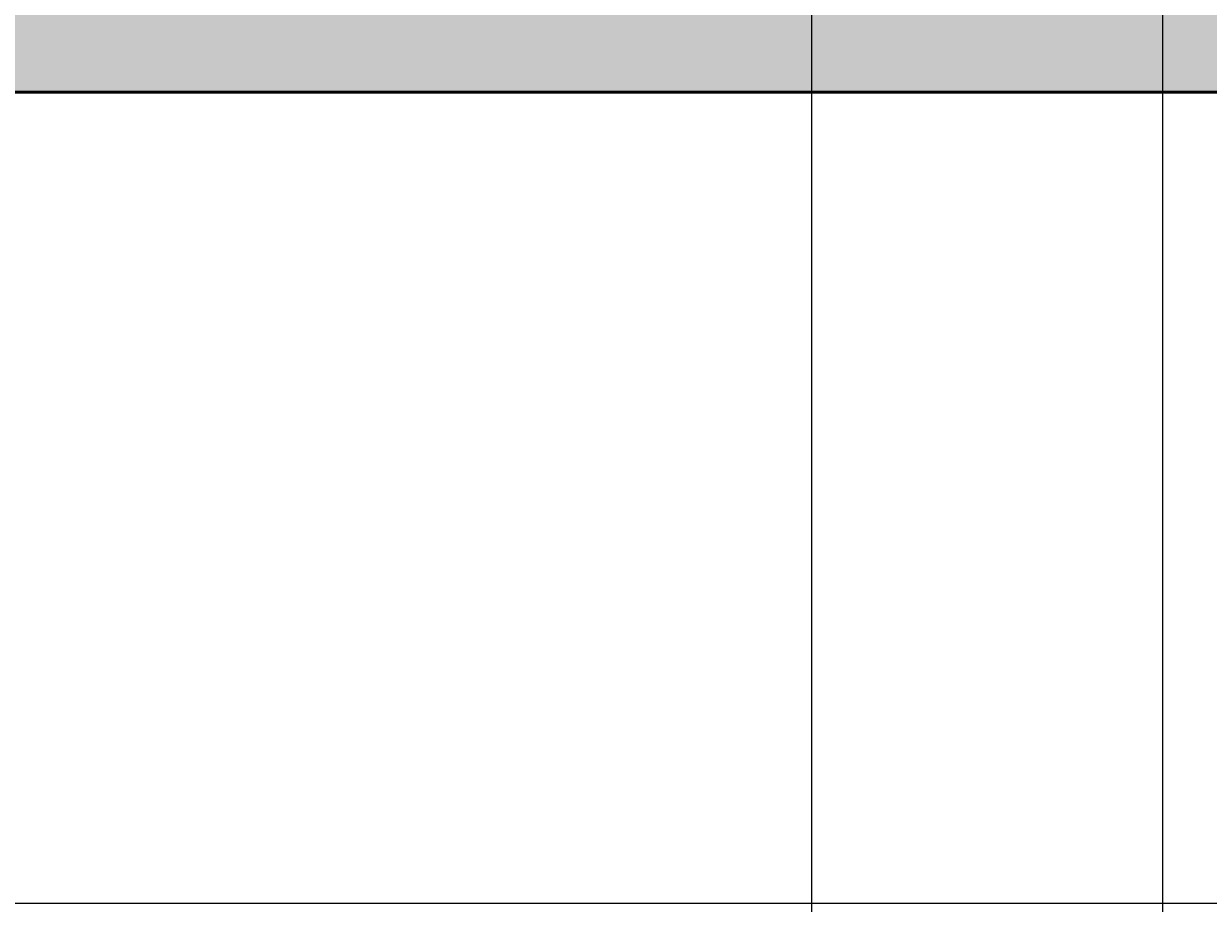
# Model space of a CAD drawing. Units: inches. Extents: x 2231 to 2461, y 2045 to 2455.
# Tile 29 of 95: x 2361 to 2396, y 2159 to 2185. Entities that reach past the tile are written whole.
import ezdxf

# ---------------------------------------------------------------- set-up
doc = ezdxf.new("R2010")
doc.units = ezdxf.units.IN
doc.layers.add('A-ANNO-DIMS', color=2, linetype='Continuous', lineweight=18)
doc.layers.add('A-WALL', color=7, linetype='Continuous', lineweight=50)
doc.layers.add('A-WALL-PATT', color=18, linetype='Continuous', lineweight=13, true_color=0x000000)
doc.styles.get("Standard").update_dxf_attribs({"font": 'arial.ttf'})
doc.dimstyles.get("Standard").update_dxf_attribs({"dimtxt": 0.18, "dimasz": 0.18, "dimexe": 0.18, "dimexo": 0.0625, "dimgap": 0.09, "dimtad": 0, "dimtih": 1, "dimtoh": 1, "dimdec": 4, "dimzin": 0, "dimdsep": 46, "dimtxsty": 'Standard', "dimcen": 0.09, "dimadec": 0, "dimazin": 0, "dimtfac": 1, "dimtdec": 4, "dimtofl": 0, "dimtmove": 0, "dimatfit": 3, "dimfxl": 1, "dimtolj": 1, "dimtzin": 0, "dimarcsym": 0})

# ---------------------------------------------------------------- blocks, each defined once
blk = doc.blocks.new('*D60')
at = {"layer": 'A-ANNO-DIMS', "color": 0, "lineweight": -2, "transparency": 16777216}
for p, q in [((2432.731, 2182.833), (2230.981, 2182.833)), ((2231.161, 2182.653), (2231.161, 2166.906)), ((2231.161, 2150.795), (2231.161, 2166.542)), ((2432.731, 2150.615), (2230.981, 2150.615))]:
    blk.add_line(p, q, dxfattribs=at)
at = {"layer": 'A-ANNO-DIMS', "color": 0, "transparency": 16777216}
for points in [[(2231.131, 2182.653), (2231.191, 2182.653), (2231.161, 2182.833)], [(2231.131, 2150.795), (2231.191, 2150.795), (2231.161, 2150.615)]]:
    blk.add_solid(points, dxfattribs=at)
at = {"layer": 'Defpoints', "color": 0, "transparency": 16777216}
for p in [(2231.161, 2182.833), (2432.794, 2182.833), (2432.794, 2150.615)]:
    blk.add_point(p, dxfattribs=at)
at = {"layer": 'A-ANNO-DIMS', "color": 0, "transparency": 16777216, "insert": (2231.161, 2166.724), "char_height": 0.18, "attachment_point": 5}
blk.add_mtext('\\A1;32.22', dxfattribs=at)
blk = doc.blocks.new('*D66')
at = {"layer": 'A-ANNO-DIMS', "color": 0, "lineweight": -2, "transparency": 16777216}
for p, q in [((2348.189, 2096.895), (2348.189, 2454.645)), ((2348.369, 2454.465), (2378.167, 2454.465)), ((2408.614, 2454.465), (2378.815, 2454.465)), ((2408.794, 2096.895), (2408.794, 2454.645))]:
    blk.add_line(p, q, dxfattribs=at)
at = {"layer": 'A-ANNO-DIMS', "color": 0, "transparency": 16777216}
for points in [[(2348.369, 2454.495), (2348.369, 2454.435), (2348.189, 2454.465)], [(2408.614, 2454.495), (2408.614, 2454.435), (2408.794, 2454.465)]]:
    blk.add_solid(points, dxfattribs=at)
at = {"layer": 'Defpoints', "color": 0, "transparency": 16777216}
for p in [(2408.794, 2454.465), (2348.189, 2096.833), (2408.794, 2096.833)]:
    blk.add_point(p, dxfattribs=at)
at = {"layer": 'A-ANNO-DIMS', "color": 0, "transparency": 16777216, "insert": (2378.491, 2454.465), "char_height": 0.18, "attachment_point": 5}
blk.add_mtext('\\A1;60.6', dxfattribs=at)
blk = doc.blocks.new('*D69')
at = {"layer": 'A-ANNO-DIMS', "color": 0, "lineweight": -2, "transparency": 16777216}
for p, q in [((2340.667, 2189.285), (2340.667, 2044.803)), ((2394.794, 2186.77), (2394.794, 2044.803)), ((2340.847, 2044.983), (2367.337, 2044.983)), ((2394.614, 2044.983), (2368.124, 2044.983))]:
    blk.add_line(p, q, dxfattribs=at)
at = {"layer": 'A-ANNO-DIMS', "color": 0, "transparency": 16777216}
for points in [[(2340.847, 2045.013), (2340.847, 2044.953), (2340.667, 2044.983)], [(2394.614, 2045.013), (2394.614, 2044.953), (2394.794, 2044.983)]]:
    blk.add_solid(points, dxfattribs=at)
at = {"layer": 'Defpoints', "color": 0, "transparency": 16777216}
for p in [(2340.667, 2189.348), (2394.794, 2186.833), (2394.794, 2044.983)]:
    blk.add_point(p, dxfattribs=at)
at = {"layer": 'A-ANNO-DIMS', "color": 0, "transparency": 16777216, "insert": (2367.73, 2044.983), "char_height": 0.18, "attachment_point": 5}
blk.add_mtext('\\A1;54.13', dxfattribs=at)
blk = doc.blocks.new('*D72')
at = {"layer": 'A-ANNO-DIMS', "color": 0, "lineweight": -2, "transparency": 16777216}
for p, q in [((2384.543, 2145.12), (2384.543, 2454.645)), ((2384.723, 2454.465), (2396.272, 2454.465)), ((2408.614, 2454.465), (2397.064, 2454.465)), ((2408.794, 2150.677), (2408.794, 2454.645))]:
    blk.add_line(p, q, dxfattribs=at)
at = {"layer": 'A-ANNO-DIMS', "color": 0, "transparency": 16777216}
for points in [[(2384.723, 2454.495), (2384.723, 2454.435), (2384.543, 2454.465)], [(2408.614, 2454.495), (2408.614, 2454.435), (2408.794, 2454.465)]]:
    blk.add_solid(points, dxfattribs=at)
at = {"layer": 'Defpoints', "color": 0, "transparency": 16777216}
for p in [(2408.794, 2454.465), (2408.794, 2150.615), (2384.543, 2145.058)]:
    blk.add_point(p, dxfattribs=at)
at = {"layer": 'A-ANNO-DIMS', "color": 0, "transparency": 16777216, "insert": (2396.668, 2454.465), "char_height": 0.18, "attachment_point": 5}
blk.add_mtext('\\A1;24.25', dxfattribs=at)
blk = doc.blocks.new('*D73')
at = {"layer": 'A-ANNO-DIMS', "color": 0, "lineweight": -2, "transparency": 16777216}
for p, q in [((2334.856, 2182.833), (2460.606, 2182.833)), ((2460.426, 2182.653), (2460.426, 2171.156)), ((2460.426, 2159.295), (2460.426, 2170.792)), ((2353.872, 2159.115), (2460.606, 2159.115))]:
    blk.add_line(p, q, dxfattribs=at)
at = {"layer": 'A-ANNO-DIMS', "color": 0, "transparency": 16777216}
for points in [[(2460.396, 2182.653), (2460.456, 2182.653), (2460.426, 2182.833)], [(2460.396, 2159.295), (2460.456, 2159.295), (2460.426, 2159.115)]]:
    blk.add_solid(points, dxfattribs=at)
at = {"layer": 'Defpoints', "color": 0, "transparency": 16777216}
for p in [(2334.794, 2182.833), (2460.426, 2182.833), (2353.809, 2159.115)]:
    blk.add_point(p, dxfattribs=at)
at = {"layer": 'A-ANNO-DIMS', "color": 0, "transparency": 16777216, "insert": (2460.426, 2170.974), "char_height": 0.18, "attachment_point": 5}
blk.add_mtext('\\A1;23.717', dxfattribs=at)

msp = doc.modelspace()

# ---------------------------------------------------------------- hatches: boundary and pattern name
at = {"layer": 'A-WALL-PATT'}
h = msp.add_hatch(color=256, dxfattribs=at)
h.dxf.hatch_style = 1
h.paths.add_polyline_path([(2441.7935, 2269.1535), (2432.7935, 2269.1535), (2432.7935, 2186.8328), (2396.7935, 2186.8328), (2396.7935, 2286.8328), (2394.7935, 2286.8328), (2394.7935, 2186.8328), (2334.7935, 2186.8328), (2334.7935, 2182.8328), (2432.7935, 2182.8328), (2432.7935, 2072.8328), (2416.6639, 2072.8328), (2416.6639, 2063.8328), (2441.7935, 2063.8328)])
h.paths.add_polyline_path([(2368.6639, 2072.8328), (2367.04, 2072.8328), (2330.7942, 2072.8328), (2330.7397, 2063.8328), (2368.6639, 2063.8328)])
h.paths.add_polyline_path([(2300.7392, 2068.3328), (2300.7392, 2072.8328), (2298.7935, 2072.8328), (2294.7935, 2072.8328), (2258.7935, 2072.8328), (2258.7935, 2120.8328), (2294.7935, 2120.8328), (2298.7935, 2120.8328), (2298.7935, 2128.8328), (2294.7935, 2128.8328), (2294.7935, 2124.8328), (2258.7935, 2124.8328), (2258.7935, 2182.8328), (2294.7935, 2182.8328), (2294.7935, 2174.8328), (2298.7935, 2174.8328), (2298.7935, 2182.8328), (2304.7935, 2182.8328), (2304.7935, 2186.8328), (2258.7935, 2186.8328), (2258.7935, 2221.999), (2249.7935, 2221.999), (2249.7935, 2063.8328), (2300.7392, 2063.8328)])
h.paths.add_polyline_path([(2391.9338, 2435.8328), (2333.82, 2435.8328), (2333.82, 2426.8328), (2368.7935, 2426.8328), (2368.7935, 2374.9508), (2368.7935, 2370.8328), (2372.3935, 2370.8328), (2372.7935, 2370.8328), (2372.7935, 2426.8328), (2391.9338, 2426.8328)])
h.paths.add_polyline_path([(2441.7935, 2435.8328), (2415.9338, 2435.8328), (2415.9338, 2426.8328), (2432.7935, 2426.8328), (2432.7935, 2334.8328), (2372.7935, 2334.8328), (2372.7935, 2346.8328), (2368.7935, 2346.8328), (2368.7935, 2306.8328), (2360.7935, 2306.8328), (2360.7935, 2302.8328), (2368.7935, 2302.8328), (2372.7935, 2302.8328), (2372.7935, 2330.8328), (2432.7935, 2330.8328), (2432.7935, 2317.1535), (2441.7935, 2317.1535)])
h.paths.add_polyline_path([(2285.82, 2435.8328), (2249.7935, 2435.8328), (2249.7935, 2269.999), (2258.7935, 2269.999), (2258.7935, 2302.8328), (2318.8168, 2302.8328), (2330.7935, 2302.8328), (2330.7935, 2306.8328), (2258.7935, 2306.8328), (2258.7935, 2426.8328), (2285.82, 2426.8328)])

# ---------------------------------------------------------------- linework, layer by layer
at = {"layer": 'A-WALL'}
msp.add_line((2334.7935, 2182.8328), (2432.7935, 2182.8328), dxfattribs=at)

# ---------------------------------------------------------------- dimensions: what is measured, and where the dimension line sits
at = {"layer": 'A-ANNO-DIMS'}
for base, p1, p2, override, picture, middle in [((2408.7935, 2454.4653), (2348.1888, 2096.8328), (2408.7935, 2096.8328), {"dimdec": 1, "dimlfac": 1, "dimrnd": 0, "dimzin": 0, "dimdsep": 46, "dimlunit": 2}, '*D66', (2378.4912, 2454.4653)), ((2408.7935, 2454.4653), (2384.5428, 2145.0576), (2408.7935, 2150.6145), {"dimdec": 2, "dimlfac": 1, "dimrnd": 0, "dimzin": 0, "dimdsep": 46, "dimlunit": 2}, '*D72', (2396.6682, 2454.4653)), ((2394.7935, 2044.9825), (2340.6673, 2189.3477), (2394.7935, 2186.8328), {"dimdec": 2, "dimlfac": 1, "dimrnd": 0, "dimzin": 0, "dimdsep": 46, "dimlunit": 2}, '*D69', (2367.7304, 2044.9825))]:
    dim = msp.add_linear_dim(base=base, p1=p1, p2=p2, dimstyle='Standard', override=override, dxfattribs=at)
    dim.commit()
    dim.dimension.update_dxf_attribs({"geometry": picture, "text_midpoint": middle})
for base, p1, p2, override, picture, middle in [((2231.161, 2182.8328), (2432.7935, 2150.6145), (2432.7935, 2182.8328), {"dimdec": 2, "dimlfac": 1, "dimrnd": 0, "dimzin": 0, "dimdsep": 46, "dimlunit": 2}, '*D60', (2231.161, 2166.7237)), ((2460.426, 2182.8328), (2353.8091, 2159.1154), (2334.7935, 2182.8328), {"dimdec": 3, "dimlfac": 1, "dimrnd": 0, "dimzin": 0, "dimdsep": 46, "dimlunit": 2}, '*D73', (2460.426, 2170.9741))]:
    dim = msp.add_linear_dim(base=base, p1=p1, p2=p2, angle=90, dimstyle='Standard', override=override, dxfattribs=at)
    dim.commit()
    dim.dimension.update_dxf_attribs({"geometry": picture, "text_midpoint": middle})

doc.saveas('drawing.dxf')
